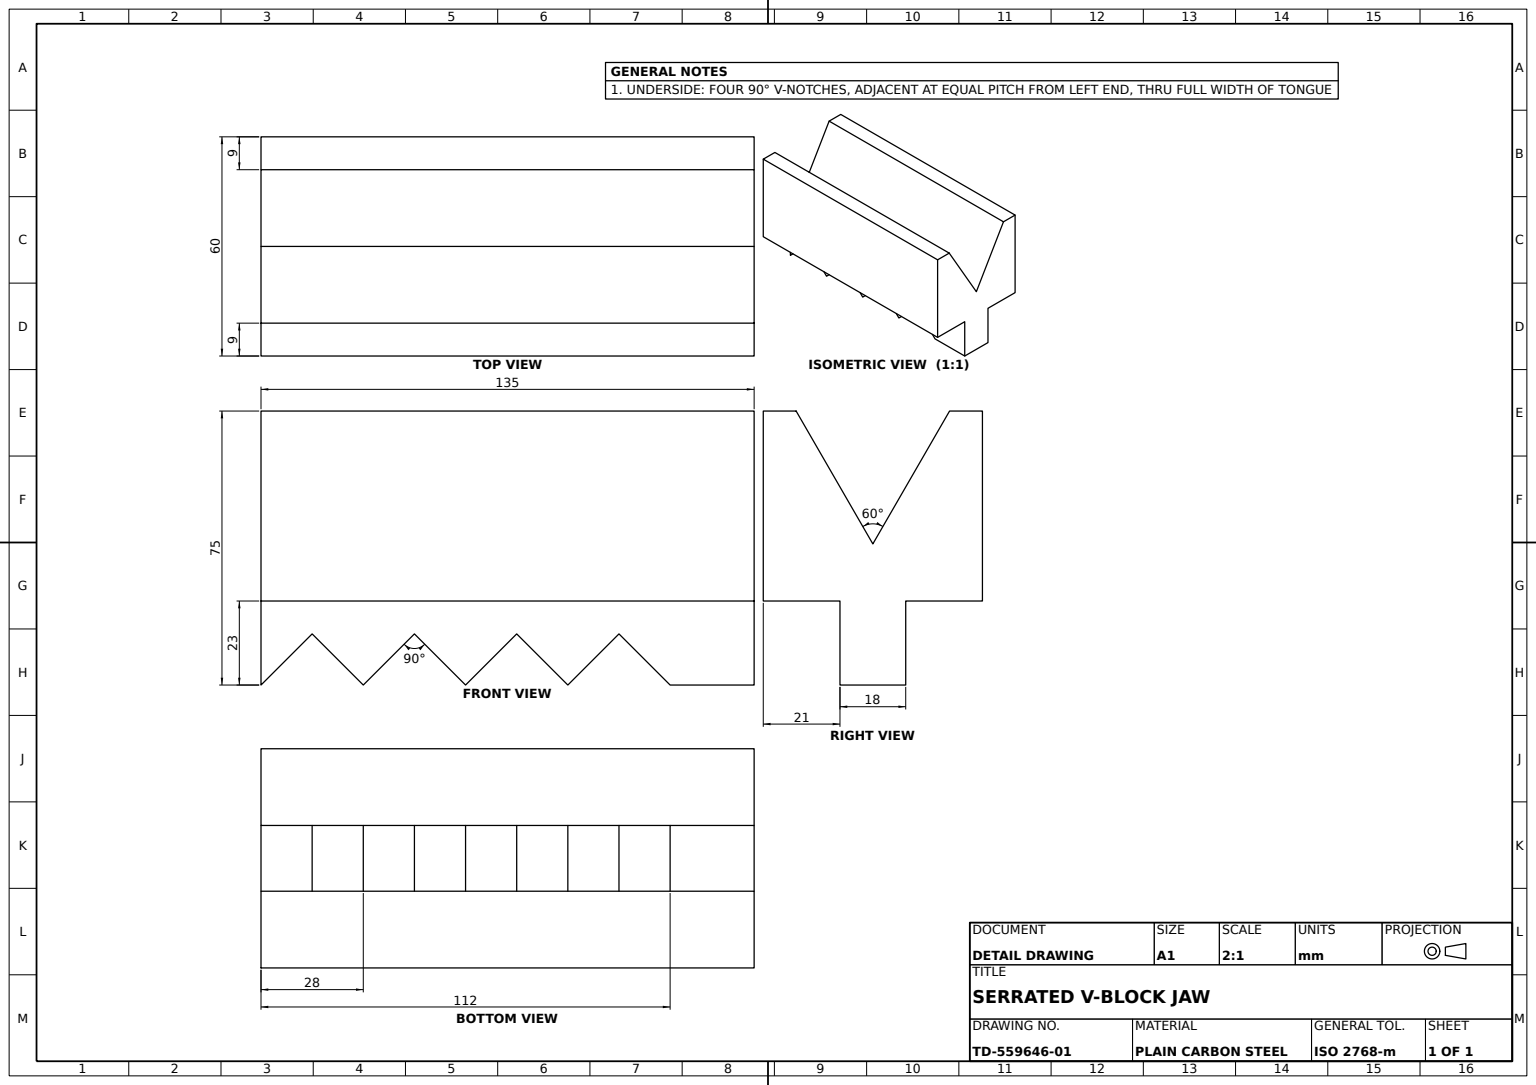
SolidWorks part; units mm, degrees
material "Plain Carbon Steel"
ref_plane "Front Plane" through (0, 0, 0) normal (0, 0, 1) x (1, 0, 0)
ref_plane "Top Plane" through (0, 0, 0) normal (0, 1, 0) x (1, 0, 0)
ref_plane "Right Plane" through (0, 0, 0) normal (1, 0, 0) x (0, 0, -1)
sketch "V-Block Profile Sketch" plane through (0, 0, 0) normal (1, 0, 0) x (0, 0, -1)
  line L0 (0, -41.2066) -> (0, 41.2066) construction
  line L1 (-30, 52) -> (-30, 0)
  line L2 (-30, 0) -> (-9, 0)
  line L3 (-9, 0) -> (-9, -23)
  line L4 (-9, -23) -> (9, -23)
  line L5 (9, -23) -> (9, 0)
  line L6 (9, 0) -> (30, 0)
  line L7 (30, 0) -> (30, 52)
  line L12 (-30, 52) -> (-21, 52)
  line L13 (-21, 52) -> (0, 15.6269)
  line L14 (0, 15.6269) -> (21, 52)
  line L15 (21, 52) -> (30, 52)
  point P4 (0, 0)
  dimension "D1" = 18
  dimension "D2" = 23
  dimension "D3" = 9
  dimension "D4" = 52
  dimension "D5" = 52
  dimension "D6" = 60
  dimension "D7" = 30
  dimension "D8" = 9
  dimension "D9" = 30
  dimension "D10" = 30
extrude "V-Block Body" add sketch "V-Block Profile Sketch" against normal blind 135
sketch "Underside Notches Sketch" plane through (0, 0, 9) normal (0, 0, 1) x (1, 0, 0)
  line L0 (-135, -23) -> (-121, -9)
  line L2 (0, 0) -> (0, -23) construction
  line L4 (-93, -9) -> (-79, -23)
  line L5 (-79, -23) -> (-65, -9)
  line L6 (-65, -9) -> (-51, -23)
  line L7 (-51, -23) -> (-37, -9)
  line L10 (-135, -23) -> (-135, -44.4296)
  line L11 (-135, -44.4296) -> (-7.6578, -38.3422)
  line L12 (-37, -9) -> (-7.6578, -38.3422)
  line L13 (-107, -23) -> (-93, -9) [skipped]
  line L14 (-121, -9) -> (-107, -23)
  line L15 (-93, -9) -> (-107, -23)
  line L16 (-135, 0) -> (0, 0) construction
  dimension "D1" = 7.6578
  dimension "D2" = 37
  dimension "D3" = 44.4296
  dimension "D4" = 4
extrude "Underside Notches Cut" cut sketch "Underside Notches Sketch" against normal blind 195
